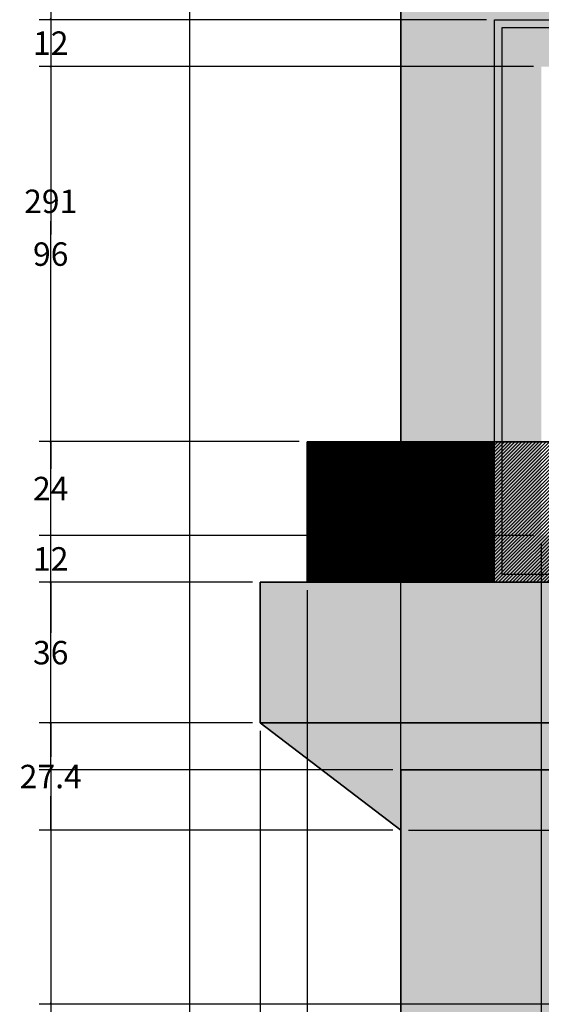
# Model space of a CAD drawing. Units: inches. Extents: x 860 to 1491, y 583 to 1370.
# Tile 4 of 8: x 865 to 998, y 839 to 1091. Entities that reach past the tile are written whole.
import ezdxf

# ---------------------------------------------------------------- set-up
doc = ezdxf.new("R2010")
doc.units = ezdxf.units.IN
doc.header["$MEASUREMENT"] = 0
doc.layers.get('0').update_dxf_attribs({"color": 250})
for name, color, linetype, lineweight in [('A-ANNO-DIMS', 2, 'Continuous', 18), ('A-ELEV', 7, 'Continuous', 35), ('A-ELEV-PATT', 9, 'Continuous', 13), ('A-GLAZ', 4, 'Continuous', 25), ('A-GLAZ-PATT', 150, 'Continuous', 13), ('A-RAIL-PATT', 150, 'Continuous', 13)]:
    doc.layers.add(name, color=color, linetype=linetype, lineweight=lineweight)
doc.styles.get("Standard").update_dxf_attribs({"font": 'arial.ttf'})
doc.dimstyles.get("Standard").update_dxf_attribs({"dimtxt": 6, "dimasz": 0.18, "dimexe": 3, "dimexo": 2, "dimgap": 2, "dimtad": 0, "dimtih": 1, "dimtoh": 1, "dimdec": 0, "dimzin": 0, "dimdsep": 46, "dimlunit": 3, "dimtxsty": 'Standard', "dimblk2": 'CLOSEDBLANK', "dimsah": 1, "dimcen": 2, "dimadec": 0, "dimazin": 0, "dimtfac": 1, "dimtdec": 0, "dimtofl": 0, "dimtmove": 0, "dimatfit": 3, "dimfxl": 1, "dimtolj": 1, "dimtzin": 0, "dimarcsym": 0})

# ---------------------------------------------------------------- blocks, each defined once
blk = doc.blocks.new('_ClosedBlank')
at = {"color": 0, "linetype": 'ByBlock', "lineweight": -2}
for p, q in [((-1, 0.17), (0, 0)), ((-1, 0.17), (-1, -0.17)), ((0, 0), (-1, -0.17))]:
    blk.add_line(p, q, dxfattribs=at)
blk = doc.blocks.new('*D2')
at = {"layer": 'A-ANNO-DIMS', "color": 0, "lineweight": -2, "transparency": 16777216}
for p, q in [((1442.44, 1328.76), (1442.44, 584.11)), ((908.34, 740.76), (908.34, 584.11)), ((908.52, 587.11), (1163.85, 587.11)), ((1442.26, 587.11), (1186.93, 587.11))]:
    blk.add_line(p, q, dxfattribs=at)
at = {"layer": 'A-ANNO-DIMS', "color": 0, "transparency": 16777216}
blk.add_solid([(908.52, 587.14), (908.52, 587.08), (908.34, 587.11)], dxfattribs=at)
at = {"layer": 'Defpoints', "color": 0, "transparency": 16777216}
for p in [(1442.44, 1330.76), (908.34, 742.76), (1442.44, 587.11)]:
    blk.add_point(p, dxfattribs=at)
at = {"layer": 'A-ANNO-DIMS', "color": 0, "lineweight": -2, "transparency": 16777216, "xscale": 0.18, "yscale": 0.18, "zscale": 0.18}
blk.add_blockref('_ClosedBlank', (1442.44, 587.11), dxfattribs=at)
at = {"layer": 'A-ANNO-DIMS', "color": 0, "transparency": 16777216, "insert": (1175.39, 587.11), "char_height": 6, "attachment_point": 5}
blk.add_mtext('\\A1;534.1', dxfattribs=at)
blk = doc.blocks.new('*D4')
at = {"layer": 'A-ANNO-DIMS', "color": 0, "lineweight": -2, "transparency": 16777216}
for p, q in [((960.34, 898.76), (869.69, 898.76)), ((872.69, 898.58), (872.69, 765.82)), ((872.69, 622.94), (872.69, 755.69)), ((906.34, 622.76), (869.69, 622.76))]:
    blk.add_line(p, q, dxfattribs=at)
at = {"layer": 'A-ANNO-DIMS', "color": 0, "transparency": 16777216}
blk.add_solid([(872.66, 622.94), (872.72, 622.94), (872.69, 622.76)], dxfattribs=at)
at = {"layer": 'Defpoints', "color": 0, "transparency": 16777216}
for p in [(872.69, 898.76), (962.34, 898.76), (908.34, 622.76)]:
    blk.add_point(p, dxfattribs=at)
at = {"layer": 'A-ANNO-DIMS', "color": 0, "lineweight": -2, "transparency": 16777216, "xscale": 0.18, "yscale": 0.18, "zscale": 0.18, "rotation": 90}
blk.add_blockref('_ClosedBlank', (872.69, 898.76), dxfattribs=at)
at = {"layer": 'A-ANNO-DIMS', "color": 0, "transparency": 16777216, "insert": (872.69, 760.76), "char_height": 6, "attachment_point": 5}
blk.add_mtext('\\A1;276', dxfattribs=at)
blk = doc.blocks.new('*D5')
at = {"layer": 'A-ANNO-DIMS', "color": 0, "lineweight": -2, "transparency": 16777216}
for p, q in [((936.34, 1189.76), (869.69, 1189.76)), ((872.69, 1189.58), (872.69, 1049.32)), ((872.69, 898.94), (872.69, 1039.19)), ((960.34, 898.76), (869.69, 898.76))]:
    blk.add_line(p, q, dxfattribs=at)
at = {"layer": 'A-ANNO-DIMS', "color": 0, "transparency": 16777216}
blk.add_solid([(872.66, 898.94), (872.72, 898.94), (872.69, 898.76)], dxfattribs=at)
at = {"layer": 'Defpoints', "color": 0, "transparency": 16777216}
for p in [(872.69, 1189.76), (938.34, 1189.76), (962.34, 898.76)]:
    blk.add_point(p, dxfattribs=at)
at = {"layer": 'A-ANNO-DIMS', "color": 0, "lineweight": -2, "transparency": 16777216, "xscale": 0.18, "yscale": 0.18, "zscale": 0.18, "rotation": 90}
blk.add_blockref('_ClosedBlank', (872.69, 1189.76), dxfattribs=at)
at = {"layer": 'A-ANNO-DIMS', "color": 0, "transparency": 16777216, "insert": (872.69, 1044.26), "char_height": 6, "attachment_point": 5}
blk.add_mtext('\\A1;291', dxfattribs=at)
blk = doc.blocks.new('*D20')
at = {"layer": 'A-ANNO-DIMS', "color": 0, "lineweight": -2, "transparency": 16777216}
for p, q in [((908.34, 744.76), (908.34, 1369.41)), ((962.34, 732.76), (962.34, 1369.41)), ((908.52, 1366.41), (929.06, 1366.41)), ((962.16, 1366.41), (941.63, 1366.41))]:
    blk.add_line(p, q, dxfattribs=at)
at = {"layer": 'A-ANNO-DIMS', "color": 0, "transparency": 16777216}
blk.add_solid([(908.52, 1366.44), (908.52, 1366.38), (908.34, 1366.41)], dxfattribs=at)
at = {"layer": 'Defpoints', "color": 0, "transparency": 16777216}
for p in [(962.34, 1366.41), (908.34, 742.76), (962.34, 730.76)]:
    blk.add_point(p, dxfattribs=at)
at = {"layer": 'A-ANNO-DIMS', "color": 0, "lineweight": -2, "transparency": 16777216, "xscale": 0.18, "yscale": 0.18, "zscale": 0.18}
blk.add_blockref('_ClosedBlank', (962.34, 1366.41), dxfattribs=at)
at = {"layer": 'A-ANNO-DIMS', "color": 0, "transparency": 16777216, "insert": (935.34, 1366.41), "char_height": 6, "attachment_point": 5}
blk.add_mtext('\\A1;54', dxfattribs=at)
blk = doc.blocks.new('*D21')
at = {"layer": 'A-ANNO-DIMS', "color": 0, "lineweight": -2, "transparency": 16777216}
for p, q in [((962.34, 732.76), (962.34, 1369.41)), ((1034.46, 828.76), (1034.46, 1369.41)), ((962.52, 1366.41), (986.33, 1366.41)), ((1034.28, 1366.41), (1010.47, 1366.41))]:
    blk.add_line(p, q, dxfattribs=at)
at = {"layer": 'A-ANNO-DIMS', "color": 0, "transparency": 16777216}
blk.add_solid([(962.52, 1366.44), (962.52, 1366.38), (962.34, 1366.41)], dxfattribs=at)
at = {"layer": 'Defpoints', "color": 0, "transparency": 16777216}
for p in [(1034.46, 1366.41), (1034.46, 826.76), (962.34, 730.76)]:
    blk.add_point(p, dxfattribs=at)
at = {"layer": 'A-ANNO-DIMS', "color": 0, "lineweight": -2, "transparency": 16777216, "xscale": 0.18, "yscale": 0.18, "zscale": 0.18}
blk.add_blockref('_ClosedBlank', (1034.46, 1366.41), dxfattribs=at)
at = {"layer": 'A-ANNO-DIMS', "color": 0, "transparency": 16777216, "insert": (998.4, 1366.41), "char_height": 6, "attachment_point": 5}
blk.add_mtext('\\A1;72.12', dxfattribs=at)
blk = doc.blocks.new('*D35')
at = {"layer": 'A-ANNO-DIMS', "color": 0, "lineweight": -2, "transparency": 16777216}
for p, q in [((1116.440309, 838.755507), (869.690309, 838.755507)), ((872.690309, 838.935507), (872.690309, 839.115507)), ((1032.458453, 826.755507), (869.690309, 826.755507)), ((872.690309, 826.575507), (872.690309, 826.395507))]:
    blk.add_line(p, q, dxfattribs=at)
at = {"layer": 'A-ANNO-DIMS', "color": 0, "transparency": 16777216}
blk.add_solid([(872.660309, 826.575507), (872.720309, 826.575507), (872.690309, 826.755507)], dxfattribs=at)
at = {"layer": 'Defpoints', "color": 0, "transparency": 16777216}
for p in [(872.690309, 838.755507), (1118.440309, 838.755507), (1034.458453, 826.755507)]:
    blk.add_point(p, dxfattribs=at)
at = {"layer": 'A-ANNO-DIMS', "color": 0, "lineweight": -2, "transparency": 16777216, "xscale": 0.18, "yscale": 0.18, "zscale": 0.18, "rotation": 270}
blk.add_blockref('_ClosedBlank', (872.690309, 838.755507), dxfattribs=at)
at = {"layer": 'A-ANNO-DIMS', "color": 0, "transparency": 16777216, "insert": (872.690309, 832.755507), "char_height": 6, "attachment_point": 5}
blk.add_mtext('\\A1;12', dxfattribs=at)
blk = doc.blocks.new('*D39')
at = {"layer": 'A-ANNO-DIMS', "color": 0, "lineweight": -2, "transparency": 16777216}
for p, q in [((924.34, 910.76), (869.69, 910.76)), ((872.69, 910.58), (872.69, 902.07)), ((872.69, 883.53), (872.69, 892.04)), ((960.34, 883.35), (869.69, 883.35))]:
    blk.add_line(p, q, dxfattribs=at)
at = {"layer": 'A-ANNO-DIMS', "color": 0, "transparency": 16777216}
blk.add_solid([(872.66, 883.53), (872.72, 883.53), (872.69, 883.35)], dxfattribs=at)
at = {"layer": 'Defpoints', "color": 0, "transparency": 16777216}
for p in [(872.69, 910.76), (926.34, 910.76), (962.34, 883.35)]:
    blk.add_point(p, dxfattribs=at)
at = {"layer": 'A-ANNO-DIMS', "color": 0, "lineweight": -2, "transparency": 16777216, "xscale": 0.18, "yscale": 0.18, "zscale": 0.18, "rotation": 90}
blk.add_blockref('_ClosedBlank', (872.69, 910.76), dxfattribs=at)
at = {"layer": 'A-ANNO-DIMS', "color": 0, "transparency": 16777216, "insert": (872.69, 897.05), "char_height": 6, "attachment_point": 5}
blk.add_mtext('\\A1;27.4', dxfattribs=at)
blk = doc.blocks.new('*D40')
at = {"layer": 'A-ANNO-DIMS', "color": 0, "lineweight": -2, "transparency": 16777216}
for p, q in [((924.34, 946.76), (869.69, 946.76)), ((872.69, 946.58), (872.69, 933.82)), ((872.69, 910.94), (872.69, 923.69)), ((924.34, 910.76), (869.69, 910.76))]:
    blk.add_line(p, q, dxfattribs=at)
at = {"layer": 'A-ANNO-DIMS', "color": 0, "transparency": 16777216}
blk.add_solid([(872.66, 910.94), (872.72, 910.94), (872.69, 910.76)], dxfattribs=at)
at = {"layer": 'Defpoints', "color": 0, "transparency": 16777216}
for p in [(872.69, 946.76), (926.34, 946.76), (926.34, 910.76)]:
    blk.add_point(p, dxfattribs=at)
at = {"layer": 'A-ANNO-DIMS', "color": 0, "lineweight": -2, "transparency": 16777216, "xscale": 0.18, "yscale": 0.18, "zscale": 0.18, "rotation": 90}
blk.add_blockref('_ClosedBlank', (872.69, 946.76), dxfattribs=at)
at = {"layer": 'A-ANNO-DIMS', "color": 0, "transparency": 16777216, "insert": (872.69, 928.76), "char_height": 6, "attachment_point": 5}
blk.add_mtext('\\A1;36', dxfattribs=at)
blk = doc.blocks.new('*D41')
at = {"layer": 'A-ANNO-DIMS', "color": 0, "lineweight": -2, "transparency": 16777216}
for p, q in [((996.340309, 958.755507), (869.690309, 958.755507)), ((872.690309, 958.935507), (872.690309, 959.115507)), ((924.340309, 946.755507), (869.690309, 946.755507)), ((872.690309, 946.575507), (872.690309, 946.395507))]:
    blk.add_line(p, q, dxfattribs=at)
at = {"layer": 'A-ANNO-DIMS', "color": 0, "transparency": 16777216}
blk.add_solid([(872.660309, 946.575507), (872.720309, 946.575507), (872.690309, 946.755507)], dxfattribs=at)
at = {"layer": 'Defpoints', "color": 0, "transparency": 16777216}
for p in [(872.690309, 958.755507), (998.340309, 958.755507), (926.340309, 946.755507)]:
    blk.add_point(p, dxfattribs=at)
at = {"layer": 'A-ANNO-DIMS', "color": 0, "lineweight": -2, "transparency": 16777216, "xscale": 0.18, "yscale": 0.18, "zscale": 0.18, "rotation": 270}
blk.add_blockref('_ClosedBlank', (872.690309, 958.755507), dxfattribs=at)
at = {"layer": 'A-ANNO-DIMS', "color": 0, "transparency": 16777216, "insert": (872.690309, 952.755507), "char_height": 6, "attachment_point": 5}
blk.add_mtext('\\A1;12', dxfattribs=at)
blk = doc.blocks.new('*D42')
at = {"layer": 'A-ANNO-DIMS', "color": 0, "lineweight": -2, "transparency": 16777216}
for p, q in [((936.34, 982.76), (869.69, 982.76)), ((872.69, 982.58), (872.69, 975.77)), ((872.69, 958.94), (872.69, 965.74)), ((996.34, 958.76), (869.69, 958.76))]:
    blk.add_line(p, q, dxfattribs=at)
at = {"layer": 'A-ANNO-DIMS', "color": 0, "transparency": 16777216}
blk.add_solid([(872.66, 958.94), (872.72, 958.94), (872.69, 958.76)], dxfattribs=at)
at = {"layer": 'Defpoints', "color": 0, "transparency": 16777216}
for p in [(872.69, 982.76), (938.34, 982.76), (998.34, 958.76)]:
    blk.add_point(p, dxfattribs=at)
at = {"layer": 'A-ANNO-DIMS', "color": 0, "lineweight": -2, "transparency": 16777216, "xscale": 0.18, "yscale": 0.18, "zscale": 0.18, "rotation": 90}
blk.add_blockref('_ClosedBlank', (872.69, 982.76), dxfattribs=at)
at = {"layer": 'A-ANNO-DIMS', "color": 0, "transparency": 16777216, "insert": (872.69, 970.76), "char_height": 6, "attachment_point": 5}
blk.add_mtext('\\A1;24', dxfattribs=at)
blk = doc.blocks.new('*D43')
at = {"layer": 'A-ANNO-DIMS', "color": 0, "lineweight": -2, "transparency": 16777216}
for p, q in [((996.34, 1078.76), (869.69, 1078.76)), ((872.69, 1078.58), (872.69, 1035.82)), ((872.69, 982.94), (872.69, 1025.69)), ((936.34, 982.76), (869.69, 982.76))]:
    blk.add_line(p, q, dxfattribs=at)
at = {"layer": 'A-ANNO-DIMS', "color": 0, "transparency": 16777216}
blk.add_solid([(872.66, 982.94), (872.72, 982.94), (872.69, 982.76)], dxfattribs=at)
at = {"layer": 'Defpoints', "color": 0, "transparency": 16777216}
for p in [(872.69, 1078.76), (998.34, 1078.76), (938.34, 982.76)]:
    blk.add_point(p, dxfattribs=at)
at = {"layer": 'A-ANNO-DIMS', "color": 0, "lineweight": -2, "transparency": 16777216, "xscale": 0.18, "yscale": 0.18, "zscale": 0.18, "rotation": 90}
blk.add_blockref('_ClosedBlank', (872.69, 1078.76), dxfattribs=at)
at = {"layer": 'A-ANNO-DIMS', "color": 0, "transparency": 16777216, "insert": (872.69, 1030.76), "char_height": 6, "attachment_point": 5}
blk.add_mtext('\\A1;96', dxfattribs=at)
blk = doc.blocks.new('*D44')
at = {"layer": 'A-ANNO-DIMS', "color": 0, "lineweight": -2, "transparency": 16777216}
for p, q in [((984.340309, 1090.755507), (869.690309, 1090.755507)), ((872.690309, 1090.935507), (872.690309, 1091.115507)), ((996.340309, 1078.755507), (869.690309, 1078.755507)), ((872.690309, 1078.575507), (872.690309, 1078.395507))]:
    blk.add_line(p, q, dxfattribs=at)
at = {"layer": 'A-ANNO-DIMS', "color": 0, "transparency": 16777216}
blk.add_solid([(872.660309, 1078.575507), (872.720309, 1078.575507), (872.690309, 1078.755507)], dxfattribs=at)
at = {"layer": 'Defpoints', "color": 0, "transparency": 16777216}
for p in [(872.690309, 1090.755507), (986.340309, 1090.755507), (998.340309, 1078.755507)]:
    blk.add_point(p, dxfattribs=at)
at = {"layer": 'A-ANNO-DIMS', "color": 0, "lineweight": -2, "transparency": 16777216, "xscale": 0.18, "yscale": 0.18, "zscale": 0.18, "rotation": 270}
blk.add_blockref('_ClosedBlank', (872.690309, 1090.755507), dxfattribs=at)
at = {"layer": 'A-ANNO-DIMS', "color": 0, "transparency": 16777216, "insert": (872.690309, 1084.755507), "char_height": 6, "attachment_point": 5}
blk.add_mtext('\\A1;12', dxfattribs=at)
blk = doc.blocks.new('*D48')
at = {"layer": 'A-ANNO-DIMS', "color": 0, "lineweight": -2, "transparency": 16777216}
for p, q in [((1222.44, 898.76), (1481.09, 898.76)), ((1478.09, 898.58), (1478.09, 896.12)), ((1478.09, 883.53), (1478.09, 885.99)), ((964.34, 883.35), (1481.09, 883.35))]:
    blk.add_line(p, q, dxfattribs=at)
at = {"layer": 'A-ANNO-DIMS', "color": 0, "transparency": 16777216}
blk.add_solid([(1478.06, 883.53), (1478.12, 883.53), (1478.09, 883.35)], dxfattribs=at)
at = {"layer": 'Defpoints', "color": 0, "transparency": 16777216}
for p in [(1220.44, 898.76), (1478.09, 898.76), (962.34, 883.35)]:
    blk.add_point(p, dxfattribs=at)
at = {"layer": 'A-ANNO-DIMS', "color": 0, "lineweight": -2, "transparency": 16777216, "xscale": 0.18, "yscale": 0.18, "zscale": 0.18, "rotation": 90}
blk.add_blockref('_ClosedBlank', (1478.09, 898.76), dxfattribs=at)
at = {"layer": 'A-ANNO-DIMS', "color": 0, "transparency": 16777216, "insert": (1478.09, 891.05), "char_height": 6, "attachment_point": 5}
blk.add_mtext('\\A1;15.402', dxfattribs=at)
blk = doc.blocks.new('*D62')
at = {"layer": 'A-ANNO-DIMS', "color": 0, "lineweight": -2, "transparency": 16777216}
for p, q in [((938.340309, 944.755507), (938.340309, 584.105507)), ((926.340309, 908.755507), (926.340309, 584.105507)), ((926.160309, 587.105507), (925.980309, 587.105507)), ((938.520309, 587.105507), (938.700309, 587.105507))]:
    blk.add_line(p, q, dxfattribs=at)
at = {"layer": 'A-ANNO-DIMS', "color": 0, "transparency": 16777216}
blk.add_solid([(926.160309, 587.135507), (926.160309, 587.075507), (926.340309, 587.105507)], dxfattribs=at)
at = {"layer": 'Defpoints', "color": 0, "transparency": 16777216}
for p in [(938.340309, 946.755507), (926.340309, 910.755507), (938.340309, 587.105507)]:
    blk.add_point(p, dxfattribs=at)
at = {"layer": 'A-ANNO-DIMS', "color": 0, "lineweight": -2, "transparency": 16777216, "xscale": 0.18, "yscale": 0.18, "zscale": 0.18, "rotation": 180}
blk.add_blockref('_ClosedBlank', (938.340309, 587.105507), dxfattribs=at)
at = {"layer": 'A-ANNO-DIMS', "color": 0, "transparency": 16777216, "insert": (932.340309, 587.105507), "char_height": 6, "attachment_point": 5}
blk.add_mtext('\\A1;12', dxfattribs=at)
blk = doc.blocks.new('*D63')
at = {"layer": 'A-ANNO-DIMS', "color": 0, "lineweight": -2, "transparency": 16777216}
for p, q in [((938.34, 944.76), (938.34, 584.11)), ((962.34, 881.35), (962.34, 584.11)), ((938.52, 587.11), (944, 587.11)), ((962.16, 587.11), (956.68, 587.11))]:
    blk.add_line(p, q, dxfattribs=at)
at = {"layer": 'A-ANNO-DIMS', "color": 0, "transparency": 16777216}
blk.add_solid([(938.52, 587.14), (938.52, 587.08), (938.34, 587.11)], dxfattribs=at)
at = {"layer": 'Defpoints', "color": 0, "transparency": 16777216}
for p in [(938.34, 946.76), (962.34, 883.35), (962.34, 587.11)]:
    blk.add_point(p, dxfattribs=at)
at = {"layer": 'A-ANNO-DIMS', "color": 0, "lineweight": -2, "transparency": 16777216, "xscale": 0.18, "yscale": 0.18, "zscale": 0.18}
blk.add_blockref('_ClosedBlank', (962.34, 587.11), dxfattribs=at)
at = {"layer": 'A-ANNO-DIMS', "color": 0, "transparency": 16777216, "insert": (950.34, 587.11), "char_height": 6, "attachment_point": 5}
blk.add_mtext('\\A1;24', dxfattribs=at)
blk = doc.blocks.new('*D64')
at = {"layer": 'A-ANNO-DIMS', "color": 0, "lineweight": -2, "transparency": 16777216}
for p, q in [((998.34, 956.76), (998.34, 584.11)), ((962.34, 881.35), (962.34, 584.11)), ((962.52, 587.11), (974.05, 587.11)), ((998.16, 587.11), (986.63, 587.11))]:
    blk.add_line(p, q, dxfattribs=at)
at = {"layer": 'A-ANNO-DIMS', "color": 0, "transparency": 16777216}
blk.add_solid([(962.52, 587.14), (962.52, 587.08), (962.34, 587.11)], dxfattribs=at)
at = {"layer": 'Defpoints', "color": 0, "transparency": 16777216}
for p in [(998.34, 958.76), (962.34, 883.35), (998.34, 587.11)]:
    blk.add_point(p, dxfattribs=at)
at = {"layer": 'A-ANNO-DIMS', "color": 0, "lineweight": -2, "transparency": 16777216, "xscale": 0.18, "yscale": 0.18, "zscale": 0.18}
blk.add_blockref('_ClosedBlank', (998.34, 587.11), dxfattribs=at)
at = {"layer": 'A-ANNO-DIMS', "color": 0, "transparency": 16777216, "insert": (980.34, 587.11), "char_height": 6, "attachment_point": 5}
blk.add_mtext('\\A1;36', dxfattribs=at)
blk = doc.blocks.new('*D65')
at = {"layer": 'A-ANNO-DIMS', "color": 0, "lineweight": -2, "transparency": 16777216}
for p, q in [((998.34, 956.76), (998.34, 584.11)), ((1079.34, 956.76), (1079.34, 584.11)), ((998.52, 587.11), (1033.12, 587.11)), ((1079.16, 587.11), (1044.56, 587.11))]:
    blk.add_line(p, q, dxfattribs=at)
at = {"layer": 'A-ANNO-DIMS', "color": 0, "transparency": 16777216}
blk.add_solid([(998.52, 587.14), (998.52, 587.08), (998.34, 587.11)], dxfattribs=at)
at = {"layer": 'Defpoints', "color": 0, "transparency": 16777216}
for p in [(998.34, 958.76), (1079.34, 958.76), (1079.34, 587.11)]:
    blk.add_point(p, dxfattribs=at)
at = {"layer": 'A-ANNO-DIMS', "color": 0, "lineweight": -2, "transparency": 16777216, "xscale": 0.18, "yscale": 0.18, "zscale": 0.18}
blk.add_blockref('_ClosedBlank', (1079.34, 587.11), dxfattribs=at)
at = {"layer": 'A-ANNO-DIMS', "color": 0, "transparency": 16777216, "insert": (1038.84, 587.11), "char_height": 6, "attachment_point": 5}
blk.add_mtext('\\A1;81', dxfattribs=at)

msp = doc.modelspace()

# ---------------------------------------------------------------- hatches: boundary and pattern name
at = {"layer": 'A-ELEV-PATT'}
h = msp.add_hatch(color=256, dxfattribs=at)
h.dxf.hatch_style = 1
h.paths.add_polyline_path([(1442.4403, 1330.7555), (1370.4403, 1330.7555), (1370.4403, 622.7555), (1442.4403, 622.7555)])
h.paths.add_polyline_path([(1358.4403, 1306.7555), (1190.4403, 1306.7555), (1190.4403, 1288.7555), (1358.4403, 1288.7555)])
h.paths.add_polyline_path([(1190.4403, 1234.7555), (962.3403, 1234.7555), (962.3403, 1198.7555), (1202.4403, 1198.7555), (1202.4403, 1216.7555), (1190.4403, 1216.7555)])
h.paths.add_polyline_path([(1202.4403, 1117.6207), (962.3403, 1117.6207), (962.3403, 982.7555), (986.3403, 982.7555), (986.3403, 1090.7555), (1178.3403, 1090.7555), (1178.3403, 982.7555), (1202.4403, 982.7555)])
h.paths.add_polyline_path([(1319.4403, 1184.7555), (1202.4403, 1184.7555), (1202.4403, 982.7555), (1211.4403, 982.7555), (1211.4403, 946.7555), (1220.4403, 946.7555), (1220.4403, 934.7555), (1319.4403, 934.7555)])
h.paths.add_polyline_path([(1271.4403, 1160.7555), (1307.4403, 1160.7555), (1307.4403, 944.7555), (1271.4403, 944.7555)], flags=16)
h.paths.add_polyline_path([(1275.4403, 1156.7555), (1303.4403, 1156.7555), (1303.4403, 948.7555), (1275.4403, 948.7555)], flags=0)
h.paths.add_polyline_path([(1202.4403, 898.7555), (962.3403, 898.7555), (962.3403, 730.7555), (1034.4585, 730.7555), (1034.4585, 826.7555), (1070.4585, 826.7555), (1070.4585, 730.7555), (1118.4403, 730.7555), (1118.4403, 838.7555), (1178.4403, 838.7555), (1178.4403, 730.7555), (1202.4403, 730.7555)])
h.paths.add_polyline_path([(1220.4403, 946.7555), (1211.4403, 946.7555), (938.3403, 946.7555), (926.3403, 946.7555), (926.3403, 910.7555), (962.3403, 910.7555), (1220.4403, 910.7555)])
h.paths.add_polyline_path([(950.3403, 730.7555), (950.3403, 734.7555), (938.3403, 742.7555), (938.3403, 730.7555), (938.3403, 622.7555), (950.3403, 622.7555)])
h = msp.add_hatch(color=256, dxfattribs=at)
h.paths.add_polyline_path([(1176.3403, 1088.7555), (988.3403, 1088.7555), (988.3403, 982.7555), (998.3403, 982.7555), (998.3403, 1078.7555), (1079.3403, 1078.7555), (1079.3403, 982.7555), (1085.3403, 982.7555), (1085.3403, 1078.7555), (1166.3403, 1078.7555), (1166.3403, 982.7555), (1176.3403, 982.7555)])
h.paths.add_polyline_path([(1176.3403, 982.7555), (1166.3403, 982.7555), (1166.3403, 958.7555), (1085.3403, 958.7555), (1085.3403, 982.7555), (1079.3403, 982.7555), (1079.3403, 958.7555), (998.3403, 958.7555), (998.3403, 982.7555), (988.3403, 982.7555), (988.3403, 948.7555), (1176.3403, 948.7555)])
h.paths.add_polyline_path([(1307.4403, 1160.7555), (1271.4403, 1160.7555), (1271.4403, 944.7555), (1307.4403, 944.7555)])
h.paths.add_polyline_path([(1275.4403, 1156.7555), (1303.4403, 1156.7555), (1303.4403, 948.7555), (1275.4403, 948.7555)], flags=16)
h.paths.add_polyline_path([(1340.4403, 862.7555), (1268.4403, 862.7555), (1268.4403, 790.7555), (1340.4403, 790.7555)])
h.paths.add_polyline_path([(1306.4403, 794.7555), (1306.4403, 858.7555), (1336.4403, 858.7555), (1336.4403, 794.7555)], flags=16)
h.paths.add_polyline_path([(1302.4403, 794.7555), (1272.4403, 794.7555), (1272.4403, 858.7555), (1302.4403, 858.7555)], flags=16)
h.paths.add_polyline_path([(1124.4403, 832.7555), (1172.4403, 832.7555), (1172.4403, 730.7555), (1178.4403, 730.7555), (1178.4403, 838.7555), (1118.4403, 838.7555), (1118.4403, 742.7555), (1124.4403, 742.7555), (1124.4403, 766.7555)])
h.paths.add_polyline_path([(1070.4585, 826.7555), (1034.4585, 826.7555), (1034.4585, 730.7555), (1070.4585, 730.7555)])
h.paths.add_polyline_path([(1066.4585, 822.7555), (1066.4585, 734.7555), (1038.4585, 734.7555), (1038.4585, 822.7555)], flags=16)
h.paths.add_polyline_path([(1129.9403, 766.7555, 1), (1124.9403, 766.7555, 1)], flags=17)
h = msp.add_hatch(color=256, dxfattribs=at)
h.dxf.hatch_style = 1
h.paths.add_polyline_path([(1220.4403, 910.7555), (938.3403, 910.7555), (926.3403, 910.7555), (962.3403, 883.3536), (962.3403, 898.7555), (1220.4403, 898.7555)])
at = {"layer": 'A-GLAZ-PATT'}
h = msp.add_hatch(color=256, dxfattribs=at)
h.paths.add_polyline_path([(1178.3403, 982.7555), (1176.3403, 982.7555), (1176.3403, 948.7555), (988.3403, 948.7555), (988.3403, 982.7555), (986.3403, 982.7555), (986.3403, 946.7555), (1178.3403, 946.7555)])
h.paths.add_polyline_path([(1178.3403, 1090.7555), (986.3403, 1090.7555), (986.3403, 982.7555), (988.3403, 982.7555), (988.3403, 1088.7555), (1176.3403, 1088.7555), (1176.3403, 982.7555), (1178.3403, 982.7555)])
h.paths.add_polyline_path([(1124.4403, 766.7555, 1), (1130.4403, 766.7555, 1)])
h.paths.add_polyline_path([(1129.9403, 766.7555, -1), (1124.9403, 766.7555, -1)], flags=16)
at = {"layer": 'A-RAIL-PATT'}
h = msp.add_hatch(dxfattribs=at)
h.set_pattern_fill('ANSI31', color=256, style=0)
h.paths.add_polyline_path([(1211.4403, 982.7555), (1202.4403, 982.7555), (1202.4403, 946.7555), (1211.4403, 946.7555)])
h.paths.add_polyline_path([(1202.4403, 982.7555), (1178.3403, 982.7555), (1178.3403, 946.7555), (1202.4403, 946.7555)])
h.paths.add_polyline_path([(986.3403, 982.7555), (962.3403, 982.7555), (962.3403, 946.7555), (986.3403, 946.7555)])
h.paths.add_polyline_path([(962.3403, 982.7555), (938.3403, 982.7555), (962.3403, 946.7555)], flags=17)
h.paths.add_polyline_path([(938.3403, 982.7555), (938.3403, 946.7555), (962.3403, 946.7555)])
h = msp.add_hatch(dxfattribs=at)
h.set_pattern_fill('ANSI31', color=256, scale=5, style=0)
h.paths.add_polyline_path([(962.3403, 982.7555), (938.3403, 982.7555), (962.3403, 946.7555)], flags=17)
h.paths.add_polyline_path([(938.3403, 982.7555), (938.3403, 946.7555), (962.3403, 946.7555)])
h.paths.add_polyline_path([(986.3403, 982.7555), (962.3403, 982.7555), (962.3403, 946.7555), (986.3403, 946.7555)])
h.paths.add_polyline_path([(998.3403, 982.7555), (988.3403, 982.7555), (988.3403, 948.7555), (1176.3403, 948.7555), (1176.3403, 982.7555), (1166.3403, 982.7555), (1166.3403, 958.7555), (1085.3403, 958.7555), (1085.3403, 982.7555), (1079.3403, 982.7555), (1079.3403, 958.7555), (998.3403, 958.7555)], flags=17)
h.paths.add_polyline_path([(1000.3403, 982.7555), (998.3403, 982.7555), (998.3403, 958.7555), (1079.3403, 958.7555), (1079.3403, 982.7555), (1077.3403, 982.7555), (1077.3403, 960.7555), (1000.3403, 960.7555)], flags=16)
h.paths.add_polyline_path([(988.3403, 982.7555), (986.3403, 982.7555), (986.3403, 946.7555), (1178.3403, 946.7555), (1178.3403, 982.7555), (1176.3403, 982.7555), (1176.3403, 948.7555), (988.3403, 948.7555)])
h.paths.add_polyline_path([(1077.3403, 982.7555), (1000.3403, 982.7555), (1000.3403, 960.7555), (1077.3403, 960.7555)], flags=0)
h.paths.add_polyline_path([(1164.3403, 982.7555), (1087.3403, 982.7555), (1087.3403, 960.7555), (1164.3403, 960.7555)], flags=16)
h.paths.add_polyline_path([(1202.4403, 982.7555), (1178.3403, 982.7555), (1178.3403, 946.7555), (1202.4403, 946.7555)])

# ---------------------------------------------------------------- linework, layer by layer
at = {"layer": 'A-ELEV'}
for p, q in [((962.3403, 946.7555), (962.3403, 1117.6207)), ((938.3403, 982.7555), (1211.4403, 982.7555)), ((938.3403, 982.7555), (938.3403, 946.7555)), ((938.3403, 982.7555), (962.3403, 946.7555)), ((962.3403, 946.7555), (926.3403, 946.7555)), ((926.3403, 946.7555), (926.3403, 910.7555)), ((938.3403, 946.7555), (1220.4403, 946.7555)), ((926.3403, 910.7555), (962.3403, 910.7555)), ((926.3403, 910.7555), (962.3403, 883.3536)), ((938.3403, 910.7555), (1220.4403, 910.7555)), ((962.3403, 730.7555), (962.3403, 898.7555)), ((962.3403, 898.7555), (1220.4403, 898.7555))]:
    msp.add_line(p, q, dxfattribs=at)
at = {"layer": 'A-GLAZ'}
for points in [[(986.3403, 1090.7555), (1178.3403, 1090.7555), (1178.3403, 946.7555), (986.3403, 946.7555)], [(988.3403, 1088.7555), (1176.3403, 1088.7555), (1176.3403, 948.7555), (988.3403, 948.7555)]]:
    msp.add_lwpolyline(points, close=True, dxfattribs=at)

# ---------------------------------------------------------------- dimensions: what is measured, and where the dimension line sits
at = {"layer": 'A-ANNO-DIMS'}
for base, p1, p2, override, picture, middle in [((962.3403, 1366.4055), (908.3403, 742.7555), (962.3403, 730.7555), {"dimdec": 0, "dimlfac": 1, "dimrnd": 0, "dimzin": 0, "dimdsep": 46, "dimlunit": 2}, '*D20', (935.3403, 1366.4055)), ((1034.4585, 1366.4055), (962.3403, 730.7555), (1034.4585, 826.7555), {"dimdec": 2, "dimlfac": 1, "dimrnd": 0, "dimzin": 0, "dimdsep": 46, "dimlunit": 2}, '*D21', (998.3994, 1366.4055)), ((1442.4403, 587.1055), (908.3403, 742.7555), (1442.4403, 1330.7555), {"dimdec": 1, "dimlfac": 1, "dimrnd": 0, "dimzin": 0, "dimdsep": 46, "dimlunit": 2}, '*D2', (1175.3903, 587.1055)), ((998.3403, 587.1055), (962.3403, 883.3536), (998.3403, 958.7555), {"dimdec": 0, "dimlfac": 1, "dimrnd": 0, "dimzin": 0, "dimdsep": 46, "dimlunit": 2}, '*D64', (980.3403, 587.1055)), ((1079.3403, 587.1055), (998.3403, 958.7555), (1079.3403, 958.7555), {"dimdec": 0, "dimlfac": 1, "dimrnd": 0, "dimzin": 0, "dimdsep": 46, "dimlunit": 2}, '*D65', (1038.8403, 587.1055)), ((938.3403, 587.1055), (926.3403, 910.7555), (938.3403, 946.7555), {"dimdec": 0, "dimlfac": 1, "dimrnd": 0, "dimzin": 0, "dimdsep": 46, "dimlunit": 2}, '*D62', (932.3403, 587.1055)), ((962.3403, 587.1055), (938.3403, 946.7555), (962.3403, 883.3536), {"dimdec": 0, "dimlfac": 1, "dimrnd": 0, "dimzin": 0, "dimdsep": 46, "dimlunit": 2}, '*D63', (950.3403, 587.1055))]:
    dim = msp.add_linear_dim(base=base, p1=p1, p2=p2, dimstyle='Standard', override=override, dxfattribs=at)
    dim.commit()
    dim.dimension.update_dxf_attribs({"geometry": picture, "text_midpoint": middle})
for base, p1, p2, override, picture, middle in [((872.6903, 1189.7555), (962.3403, 898.7555), (938.3403, 1189.7555), {"dimdec": 0, "dimlfac": 1, "dimrnd": 0, "dimzin": 0, "dimdsep": 46, "dimlunit": 2}, '*D5', (872.6903, 1044.2555)), ((872.6903, 1090.7555), (998.3403, 1078.7555), (986.3403, 1090.7555), {"dimdec": 0, "dimlfac": 1, "dimrnd": 0, "dimzin": 0, "dimdsep": 46, "dimlunit": 2}, '*D44', (872.6903, 1084.7555)), ((872.6903, 1078.7555), (938.3403, 982.7555), (998.3403, 1078.7555), {"dimdec": 0, "dimlfac": 1, "dimrnd": 0, "dimzin": 0, "dimdsep": 46, "dimlunit": 2}, '*D43', (872.6903, 1030.7555)), ((872.6903, 982.7555), (998.3403, 958.7555), (938.3403, 982.7555), {"dimdec": 0, "dimlfac": 1, "dimrnd": 0, "dimzin": 0, "dimdsep": 46, "dimlunit": 2}, '*D42', (872.6903, 970.7555)), ((872.6903, 958.7555), (926.3403, 946.7555), (998.3403, 958.7555), {"dimdec": 0, "dimlfac": 1, "dimrnd": 0, "dimzin": 0, "dimdsep": 46, "dimlunit": 2}, '*D41', (872.6903, 952.7555)), ((872.6903, 946.7555), (926.3403, 910.7555), (926.3403, 946.7555), {"dimdec": 0, "dimlfac": 1, "dimrnd": 0, "dimzin": 0, "dimdsep": 46, "dimlunit": 2}, '*D40', (872.6903, 928.7555)), ((872.6903, 910.7555), (962.3403, 883.3536), (926.3403, 910.7555), {"dimdec": 1, "dimlfac": 1, "dimrnd": 0, "dimzin": 0, "dimdsep": 46, "dimlunit": 2}, '*D39', (872.6903, 897.0545)), ((872.6903, 898.7555), (908.3403, 622.7555), (962.3403, 898.7555), {"dimdec": 0, "dimlfac": 1, "dimrnd": 0, "dimzin": 0, "dimdsep": 46, "dimlunit": 2}, '*D4', (872.6903, 760.7555)), ((1478.0903, 898.7555), (962.3403, 883.3536), (1220.4403, 898.7555), {"dimdec": 3, "dimlfac": 1, "dimrnd": 0, "dimzin": 0, "dimdsep": 46, "dimlunit": 2}, '*D48', (1478.0903, 891.0545)), ((872.6903, 838.7555), (1034.4585, 826.7555), (1118.4403, 838.7555), {"dimdec": 0, "dimlfac": 1, "dimrnd": 0, "dimzin": 0, "dimdsep": 46, "dimlunit": 2}, '*D35', (872.6903, 832.7555))]:
    dim = msp.add_linear_dim(base=base, p1=p1, p2=p2, angle=90, dimstyle='Standard', override=override, dxfattribs=at)
    dim.commit()
    dim.dimension.update_dxf_attribs({"geometry": picture, "text_midpoint": middle})

doc.saveas('drawing.dxf')
